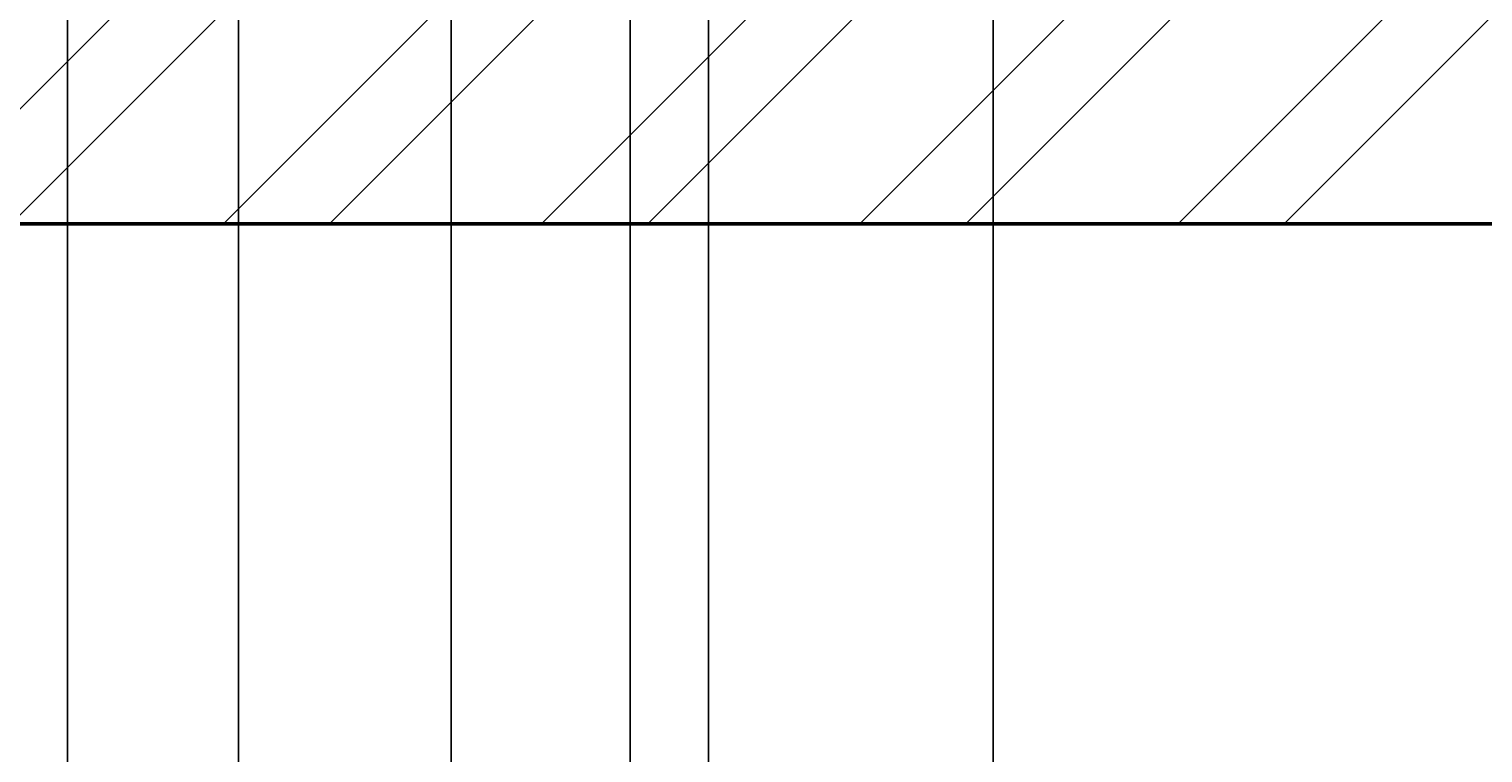
# Model space of a CAD drawing. Units: inches. Extents: x 2812 to 3051, y 1398 to 1659.
# Tile 57 of 65: x 2944 to 3005, y 1528 to 1559. Entities that reach past the tile are written whole.
import ezdxf

# ---------------------------------------------------------------- set-up
doc = ezdxf.new("R2010")
doc.units = ezdxf.units.IN
for name, color, linetype, lineweight in [('A-ANNO-DIMS', 2, 'Continuous', 18), ('S-CONC', 7, 'Continuous', 50), ('S-CONC-PATT', 8, 'Continuous', 18)]:
    doc.layers.add(name, color=color, linetype=linetype, lineweight=lineweight)
doc.styles.get("Standard").update_dxf_attribs({"font": 'arial.ttf'})
doc.dimstyles.get("Standard").update_dxf_attribs({"dimtxt": 0.18, "dimasz": 0.18, "dimexe": 0.18, "dimexo": 0.0625, "dimgap": 0.09, "dimtad": 0, "dimtih": 1, "dimtoh": 1, "dimdec": 4, "dimzin": 0, "dimdsep": 46, "dimtxsty": 'Standard', "dimcen": 0.09, "dimadec": 0, "dimazin": 0, "dimtfac": 1, "dimtdec": 4, "dimtofl": 0, "dimtmove": 0, "dimatfit": 3, "dimfxl": 1, "dimtolj": 1, "dimtzin": 0, "dimarcsym": 0})

# ---------------------------------------------------------------- blocks, each defined once
blk = doc.blocks.new('*D30')
at = {"layer": 'A-ANNO-DIMS', "color": 0, "lineweight": -2, "transparency": 16777216}
for p, q in [((2945.147, 1598.692), (2945.147, 1397.505)), ((2952.385, 1559.757), (2952.385, 1397.505)), ((2945.327, 1397.685), (2948.373, 1397.685)), ((2952.205, 1397.685), (2949.159, 1397.685))]:
    blk.add_line(p, q, dxfattribs=at)
at = {"layer": 'A-ANNO-DIMS', "color": 0, "transparency": 16777216}
for points in [[(2945.327, 1397.715), (2945.327, 1397.655), (2945.147, 1397.685)], [(2952.205, 1397.715), (2952.205, 1397.655), (2952.385, 1397.685)]]:
    blk.add_solid(points, dxfattribs=at)
at = {"layer": 'Defpoints', "color": 0, "transparency": 16777216}
for p in [(2945.147, 1598.754), (2952.385, 1559.82), (2952.385, 1397.685)]:
    blk.add_point(p, dxfattribs=at)
at = {"layer": 'A-ANNO-DIMS', "color": 0, "transparency": 16777216, "insert": (2948.766, 1397.685), "char_height": 0.18, "attachment_point": 5}
blk.add_mtext('\\A1;7.238', dxfattribs=at)
blk = doc.blocks.new('*D31')
at = {"layer": 'A-ANNO-DIMS', "color": 0, "lineweight": -2, "transparency": 16777216}
for p, q in [((2972.272, 1594.192), (2972.272, 1397.505)), ((2961.385, 1559.757), (2961.385, 1397.505)), ((2961.565, 1397.685), (2966.373, 1397.685)), ((2972.092, 1397.685), (2967.283, 1397.685))]:
    blk.add_line(p, q, dxfattribs=at)
at = {"layer": 'A-ANNO-DIMS', "color": 0, "transparency": 16777216}
for points in [[(2961.565, 1397.715), (2961.565, 1397.655), (2961.385, 1397.685)], [(2972.092, 1397.715), (2972.092, 1397.655), (2972.272, 1397.685)]]:
    blk.add_solid(points, dxfattribs=at)
at = {"layer": 'Defpoints', "color": 0, "transparency": 16777216}
for p in [(2972.272, 1594.254), (2961.385, 1559.82), (2972.272, 1397.685)]:
    blk.add_point(p, dxfattribs=at)
at = {"layer": 'A-ANNO-DIMS', "color": 0, "transparency": 16777216, "insert": (2966.828, 1397.685), "char_height": 0.18, "attachment_point": 5}
blk.add_mtext('\\A1;10.887', dxfattribs=at)
blk = doc.blocks.new('*D32')
at = {"layer": 'A-ANNO-DIMS', "color": 0, "lineweight": -2, "transparency": 16777216}
for p, q in [((2984.316, 1598.757), (2984.316, 1397.505)), ((2972.272, 1594.192), (2972.272, 1397.505)), ((2972.452, 1397.685), (2977.839, 1397.685)), ((2984.136, 1397.685), (2978.748, 1397.685))]:
    blk.add_line(p, q, dxfattribs=at)
at = {"layer": 'A-ANNO-DIMS', "color": 0, "transparency": 16777216}
for points in [[(2972.452, 1397.715), (2972.452, 1397.655), (2972.272, 1397.685)], [(2984.136, 1397.715), (2984.136, 1397.655), (2984.316, 1397.685)]]:
    blk.add_solid(points, dxfattribs=at)
at = {"layer": 'Defpoints', "color": 0, "transparency": 16777216}
for p in [(2984.316, 1598.82), (2972.272, 1594.254), (2984.316, 1397.685)]:
    blk.add_point(p, dxfattribs=at)
at = {"layer": 'A-ANNO-DIMS', "color": 0, "transparency": 16777216, "insert": (2978.294, 1397.685), "char_height": 0.18, "attachment_point": 5}
blk.add_mtext('\\A1;12.044', dxfattribs=at)
blk = doc.blocks.new('*D69')
at = {"layer": 'A-ANNO-DIMS', "color": 0, "lineweight": -2, "transparency": 16777216}
for p, q in [((2961.385, 1472.098), (2961.385, 1659.35)), ((2961.565, 1659.17), (2964.795, 1659.17)), ((2968.776, 1659.17), (2965.546, 1659.17)), ((2968.956, 1467.81), (2968.956, 1659.35))]:
    blk.add_line(p, q, dxfattribs=at)
at = {"layer": 'A-ANNO-DIMS', "color": 0, "transparency": 16777216}
for points in [[(2961.565, 1659.2), (2961.565, 1659.14), (2961.385, 1659.17)], [(2968.776, 1659.2), (2968.776, 1659.14), (2968.956, 1659.17)]]:
    blk.add_solid(points, dxfattribs=at)
at = {"layer": 'Defpoints', "color": 0, "transparency": 16777216}
for p in [(2968.956, 1659.17), (2961.385, 1472.035), (2968.956, 1467.747)]:
    blk.add_point(p, dxfattribs=at)
at = {"layer": 'A-ANNO-DIMS', "color": 0, "transparency": 16777216, "insert": (2965.17, 1659.17), "char_height": 0.18, "attachment_point": 5}
blk.add_mtext('\\A1;7.571', dxfattribs=at)

msp = doc.modelspace()

# ---------------------------------------------------------------- hatches: boundary and pattern name
at = {"layer": 'S-CONC-PATT'}
h = msp.add_hatch(dxfattribs=at)
h.set_pattern_fill('ANSI32', color=256)
h.paths.add_polyline_path([(3027.3849, 1646.82), (2835.3849, 1646.82), (2835.3849, 1603.2296), (2844.3849, 1603.2296), (2844.3849, 1637.82), (3018.3849, 1637.82), (3018.3849, 1602.5441), (3027.3849, 1602.5441)])
h.paths.add_polyline_path([(2844.3849, 1594.2296), (2835.3849, 1594.2296), (2835.3849, 1550.82), (3027.3849, 1550.82), (3027.3849, 1593.5441), (3018.3849, 1593.5441), (3018.3849, 1559.82), (2844.3849, 1559.82)])
h.paths.add_polyline_path([(2844.3849, 1482.0354), (2835.3849, 1482.0354), (2835.3849, 1463.4959), (2844.3849, 1463.4959)])
h.paths.add_polyline_path([(2844.3849, 1461.4959), (2835.3849, 1461.4959), (2835.3849, 1416.0354), (2844.3849, 1416.0354)])
h.paths.add_polyline_path([(3027.3849, 1482.0354), (3018.3849, 1482.0354), (3018.3849, 1463.2854), (3027.3849, 1463.2854)])
h.paths.add_polyline_path([(3027.3849, 1461.2854), (3018.3849, 1461.2854), (3018.3849, 1416.0354), (3027.3849, 1416.0354)])
h.paths.add_polyline_path([(2961.3849, 1448.4738), (2952.3849, 1448.4738), (2952.3849, 1416.0354), (2961.3849, 1416.0354)])
h.paths.add_polyline_path([(2961.3849, 1462.3026), (2952.3849, 1462.3026), (2952.3849, 1450.4738), (2961.3849, 1450.4738)])
h.paths.add_polyline_path([(2961.3849, 1472.0354), (2952.3849, 1472.0354), (2952.3849, 1462.3026), (2961.3849, 1462.3026)])

# ---------------------------------------------------------------- linework, layer by layer
at = {"layer": 'S-CONC'}
msp.add_line((3027.3849, 1550.82), (2835.3849, 1550.82), dxfattribs=at)

# ---------------------------------------------------------------- dimensions: what is measured, and where the dimension line sits
at = {"layer": 'A-ANNO-DIMS'}
for base, p1, p2, picture, middle in [((2968.9558, 1659.17), (2961.3849, 1472.0354), (2968.9558, 1467.7474), '*D69', (2965.1704, 1659.17)), ((2952.3849, 1397.6854), (2945.1467, 1598.7541), (2952.3849, 1559.82), '*D30', (2948.7658, 1397.6854)), ((2984.3156, 1397.6854), (2972.2716, 1594.2541), (2984.3156, 1598.82), '*D32', (2978.2936, 1397.6854)), ((2972.2716, 1397.6854), (2961.3849, 1559.82), (2972.2716, 1594.2541), '*D31', (2966.8282, 1397.6854))]:
    dim = msp.add_linear_dim(base=base, p1=p1, p2=p2, dimstyle='Standard', override={"dimdec": 3, "dimlfac": 1, "dimrnd": 0, "dimzin": 0, "dimdsep": 46, "dimlunit": 2}, dxfattribs=at)
    dim.commit()
    dim.dimension.update_dxf_attribs({"geometry": picture, "text_midpoint": middle})

doc.saveas('drawing.dxf')
